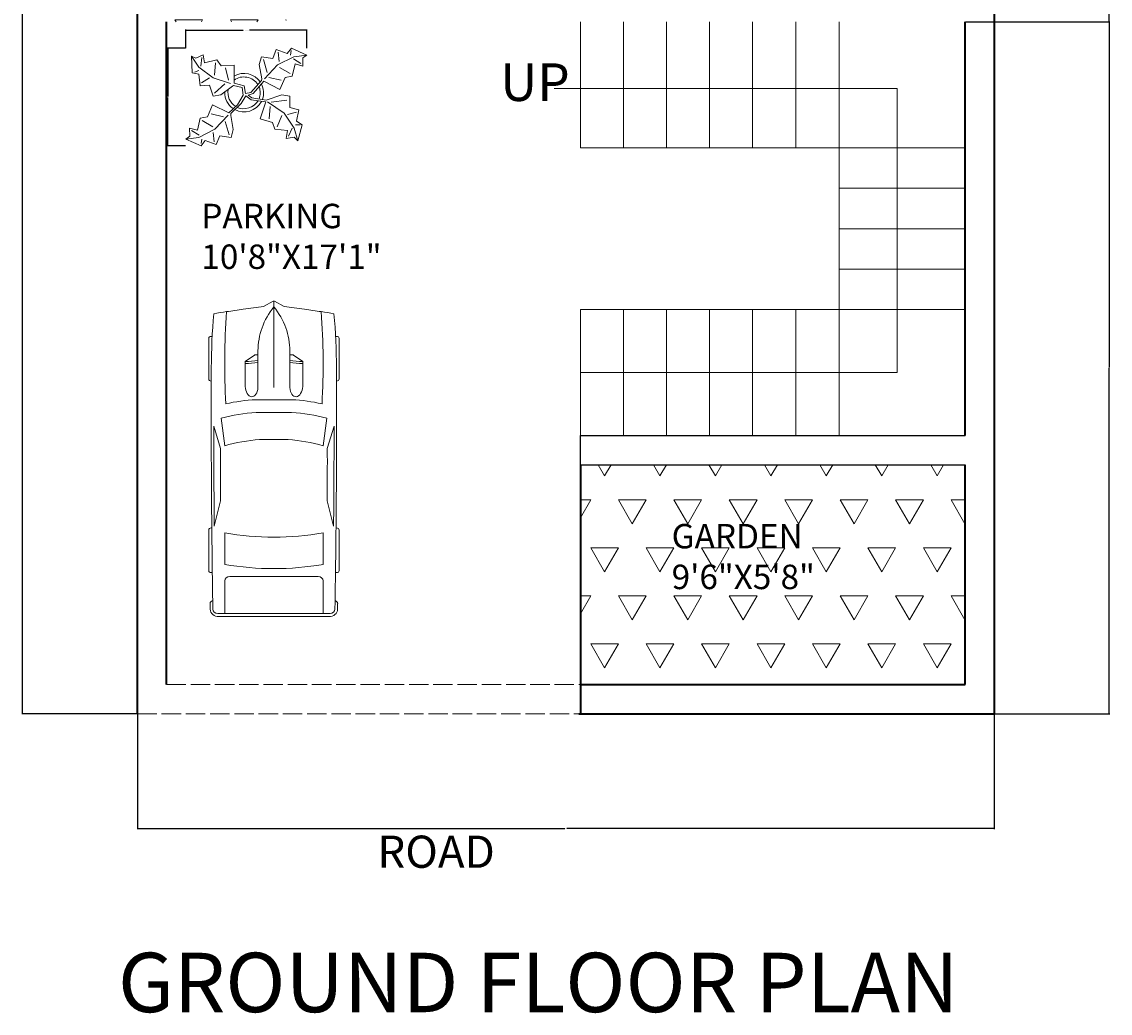
# Model space of a CAD drawing. Units: inches. Extents: x 7766 to 8631, y 9203 to 9940.
# Tile 1 of 6: x 7766 to 8103, y 9203 to 9510. Entities that reach past the tile are written whole.
import ezdxf

# ---------------------------------------------------------------- set-up
doc = ezdxf.new("R2010")
doc.units = ezdxf.units.IN
doc.linetypes.add('ACAD_ISO02W100', pattern=[15, 12, -3])
for name, color, linetype, lineweight in [('A-ANNO-DIMS', 2, 'Continuous', 18), ('A-ANNO-TEXT', 7, 'Continuous', 18), ('A-AREA-IDEN', 11, 'Continuous', 18), ('A-WALL', 7, 'Continuous', 35), ('C-SITE-ENTR', 7, 'ACAD_ISO02W100', 18), ('car', 20, 'Continuous', 13), ('floor', 7, 'Continuous', 25), ('flower', 70, 'Continuous', 18), ('L-PLNT-PATT', 60, 'Continuous', 13), ('stair', 2, 'Continuous', 18), ('TITLE', 4, 'Continuous', 35)]:
    doc.layers.add(name, color=color, linetype=linetype, lineweight=lineweight)
doc.styles.get("Standard").update_dxf_attribs({"font": 'arial.ttf'})
doc.dimstyles.get("Standard").update_dxf_attribs({"dimtxt": 0.18, "dimasz": 0.18, "dimexe": 0.18, "dimexo": 0.0625, "dimgap": 0.09, "dimtad": 0, "dimtih": 1, "dimtoh": 1, "dimdec": 4, "dimzin": 0, "dimdsep": 46, "dimtxsty": 'Standard', "dimcen": 0.09, "dimadec": 0, "dimazin": 0, "dimtfac": 1, "dimtdec": 4, "dimtofl": 0, "dimtmove": 0, "dimatfit": 3, "dimfxl": 1, "dimtolj": 1, "dimtzin": 0, "dimarcsym": 0})

# ---------------------------------------------------------------- blocks, each defined once
blk = doc.blocks.new('Plant - Rubber or Philodendron')
for p, q in [((8.8871, 10.7908), (9.9809, 13.4933)), ((9.9809, 13.4933), (13.3837, 12.301)), ((13.3837, 12.301), (14.68, 13.9039)), ((14.68, 13.9039), (19.3848, 11.8146)), ((-16.2005, 11.4774), (-13.9899, 8.1064)), ((-16.2005, 11.4774), (-14.8639, 10.7964)), ((-16.0159, 6.3329), (-16.2005, 11.4774)), ((-14.8639, 10.7964), (-12.6195, 11.8975)), ((-13.3174, 8.325), (-13.0735, 11.0065)), ((-12.6195, 11.8975), (-12.1909, 9.4345)), ((-12.1909, 9.4345), (-8.3829, 10.3)), ((-8.3829, 10.3), (-7.0549, 8.501)), ((4.6914, 8.8812), (5.3859, 11.2828)), ((5.3859, 11.2828), (8.8871, 10.7908)), ((5.9878, 10.4842), (7.1971, 6.3869)), ((15.3859, 11.3055), (10.3916, 8.7942)), ((10.5828, 12.6946), (10.8893, 9.7953)), ((14.5816, 13.2037), (14.3848, 11.8033)), ((15.2875, 10.6053), (17.5907, 9.2105)), ((19.3848, 11.8146), (15.3859, 11.3055)), ((19.3848, 11.8146), (18.1868, 10.9119)), ((18.1868, 10.9119), (18.1925, 8.4119)), ((-15.3434, 6.5514), (-13.9984, 6.9884)), ((-13.9899, 8.1064), (-9.5434, 4.7185)), ((-8.8369, 9.409), (-9.0894, 5.6095)), ((-7.0549, 8.501), (-3.0284, 8.6941)), ((-4.8529, 4.012), (-5.7184, 7.82)), ((-3.0284, 8.6941), (-3.0709, 3.1041)), ((4.6914, 8.8812), (5.5014, 4.4831)), ((10.3916, 8.7942), (6.2847, 4.4028)), ((14.2977, 6.1031), (10.9934, 7.9956)), ((15.7909, 9.1065), (14.8995, 5.3044)), ((18.1925, 8.4119), (15.7909, 9.1065)), ((-14.0069, 5.8704), (-16.0159, 6.3329)), ((-13.5868, 2.2894), (-14.0069, 5.8704)), ((-13.1329, 3.1804), (-10.6614, 4.727)), ((-9.5434, 4.7185), (-4.1917, 2.9888)), ((2.1141, 0.2298), (5.4346, 3.9146)), ((6.1032, 3.6844), (2.8262, -0.031)), ((5.4346, 3.9146), (5.5014, 4.4831)), ((11.1089, 1.1958), (6.1032, 3.6844)), ((7.7005, 4.8881), (11.5025, 3.9967)), ((12.7005, 4.8994), (11.1089, 1.1958)), ((14.8995, 5.3044), (12.7005, 4.8994)), ((-10.6784, 2.491), (-13.5868, 2.2894)), ((-9.5858, -0.8715), (-10.6784, 2.491)), ((-9.1318, 0.0195), (-5.9793, 2.9025)), ((-7.1228, -0.443), (-3.5248, 2.2131)), ((-3.5248, 2.2131), (-3.3011, 2.4355)), ((-3.3011, 2.4355), (-0.5306, 1.7947)), ((-3.0709, 3.1041), (0.0797, 2.3163)), ((-0.5306, 1.7947), (-0.2255, -0.5527)), ((-0.5306, 1.7947), (-0.5306, 1.7947)), ((0.0797, 2.3163), (0.4866, -0.031)), ((0.4866, -0.031), (2.1141, 0.2298)), ((-7.1228, -0.443), (-9.5858, -0.8715)), ((-4.0579, -6.2781), (-0.9375, -3.1608)), ((-2.019, -3.6148), (-0.2255, -0.5527)), ((-0.9375, -3.1608), (0.5883, -0.8135)), ((0.5883, -0.8135), (2.2447, -2.0916)), ((2.8262, -0.031), (1.3003, -0.5527)), ((1.3003, -0.5527), (2.4193, -1.4655)), ((2.2447, -2.0916), (6.7108, -2.6626)), ((2.4193, -1.4655), (6.895, -2.1175)), ((4.943, -7.9659), (6.7108, -2.6626)), ((11.6605, -0.5413), (6.895, -2.1175)), ((12.3677, -6.1981), (7.219, -2.6772)), ((8.3544, -2.7453), (13.1973, -2.1704)), ((11.6605, -0.5413), (14.1354, -0.8948)), ((14.1354, -0.8948), (14.1354, -4.4304)), ((-11.3237, -7.2629), (-9.7321, -3.5593)), ((-6.3237, -7.2516), (-10.1257, -6.3602)), ((-9.7321, -3.5593), (-4.7264, -6.0479)), ((-2.019, -3.6148), (-4.7264, -6.0479)), ((-4.1246, -6.8466), (-4.0579, -6.2781)), ((8.125, -4.0768), (7.7715, -7.9659)), ((15.5496, -10.7943), (12.3677, -6.1981)), ((16.2567, -5.8446), (13.4283, -6.5517)), ((14.1354, -4.4304), (16.9638, -5.1375)), ((16.9638, -5.1375), (16.2567, -8.673)), ((-14.4141, -11.4699), (-13.5228, -7.6679)), ((-13.5228, -7.6679), (-11.3237, -7.2629)), ((-12.921, -8.4665), (-9.6166, -10.359)), ((-9.0148, -11.1577), (-4.9047, -6.8122)), ((-4.611, -12.8477), (-5.8203, -8.7504)), ((-3.3146, -11.2447), (-4.1246, -6.8466)), ((8.8321, -9.0266), (4.943, -7.9659)), ((9.5392, -11.1479), (8.8321, -9.0266)), ((10.2463, -10.4408), (11.6605, -6.9053)), ((17.3174, -9.7337), (15.9032, -9.7337)), ((16.2567, -8.673), (18.0245, -9.7337)), ((18.0245, -9.7337), (16.6103, -14.6834)), ((-18.008, -14.1781), (-16.8101, -13.2754)), ((-16.8157, -10.7754), (-14.4141, -11.4699)), ((-16.8101, -13.2754), (-16.8157, -10.7754)), ((-13.9107, -12.9688), (-16.2139, -11.574)), ((-14.0091, -13.669), (-9.0148, -11.1577)), ((-9.206, -15.0581), (-9.5126, -12.1588)), ((-7.5103, -13.1543), (-8.6042, -15.8568)), ((-4.0092, -13.6463), (-7.5103, -13.1543)), ((-3.3146, -11.2447), (-4.0092, -13.6463)), ((13.4283, -11.5015), (9.5392, -11.1479)), ((13.0748, -13.9763), (13.4283, -11.5015)), ((14.8425, -10.7943), (13.7819, -13.2692)), ((16.6103, -14.6834), (15.5496, -10.7943)), ((-18.008, -14.1781), (-14.0091, -13.669)), ((-13.3032, -16.2674), (-18.008, -14.1781)), ((-12.0069, -14.6645), (-13.3032, -16.2674)), ((-13.2048, -15.5672), (-13.008, -14.1668)), ((-8.6042, -15.8568), (-12.0069, -14.6645)), ((15.5496, -13.6228), (13.0748, -13.9763)), ((16.6103, -14.6834), (15.5496, -13.6228))]:
    blk.add_line(p, q)
for centre, radius, start, end in [((0, 0), 6.1275, 34.37569, 120.1028), ((-0.0601, -0.2075), 5.2461, 33.82192, 124.9414), ((0.0308, 0.1664), 6, 178.6147, 235.1169), ((0.0308, 0.1664), 5, 168.1647, 238.6725), ((-0.2664, 0.1682), 5.2775, 338.4094, 20.03007), ((-0.098, 0.1364), 6.1288, 341.2017, 26.09184), ((-0.0234, 0.3825), 6.1492, 242.5812, 331.2714), ((-0.1102, 0.4886), 5.2883, 247.3711, 327.472)]:
    blk.add_arc(centre, radius, start, end)
blk = doc.blocks.new('*U22')
for p, q in [((21.1, 37.41), (21.1, 36.83)), ((46.55, 38.89), (22.35, 38.89)), ((47.8, 37.39), (47.8, 37.41)), ((87.99, 31.87), (74.76, 35.92)), ((134.31, 35.6), (119.29, 31.78)), ((135.45, 37.07), (135.45, 37.41)), ((136.7, 38.89), (160.9, 38.89)), ((162.15, 37.41), (162.15, 36.77)), ((186.47, -33.5), (186.47, 33.5)), ((188.4, -32.76), (188.4, 32.76)), ((70.03, 31.54), (86.41, 29.35)), ((138.42, 29.35), (157.25, 29.35)), ((164.52, 26.39), (164.52, -26.39)), ((186.47, 29.35), (167.01, 29.35)), ((32.27, 11.63), (36.13, 17.17)), ((36.13, 17.17), (50.94, 17.17)), ((29.77, 9.51), (51.68, 9.51)), ((32.12, 9.51), (32.12, 11.15)), ((58.92, -10.77), (58.92, 10.77)), ((66.55, -10.53), (66.55, 10.53)), ((82.74, 8.5), (82.74, -8.5)), ((186.47, -10.53), (186.47, 10.53)), ((3.27, 6.13), (0.1, 0.41)), ((0, 0), (51.68, 0)), ((0.1, -0.41), (3.27, -6.13)), ((29.77, -9.51), (51.68, -9.51)), ((32.12, -9.51), (32.12, -11.15)), ((32.27, -11.63), (36.13, -17.17)), ((36.13, -17.17), (50.94, -17.17)), ((86.41, -29.35), (70.03, -31.54)), ((87.99, -31.87), (74.76, -35.92)), ((134.31, -35.6), (119.29, -31.78)), ((157.25, -29.35), (138.42, -29.35)), ((167.01, -29.35), (186.47, -29.35)), ((21.1, -37.41), (21.1, -36.83)), ((46.55, -38.89), (22.35, -38.89)), ((47.8, -37.39), (47.8, -37.41)), ((135.45, -37.07), (135.45, -37.41)), ((136.7, -38.89), (160.9, -38.89)), ((162.15, -37.41), (162.15, -36.77))]:
    blk.add_line(p, q)
for centre, major_axis, ratio, start_param, end_param in [((266.03, -27.52), (0, 313.31), 0.842304, 1.367076, 1.39176), ((41.19, -490.86), (0, 528.23), 0.842304, 0.00281, 0.075598), ((22.35, 37.41), (0, -1.48), 0.842304, 3.141593, 4.712389), ((64.48, -10555.62), (0, 10593.03), 0.842304, -0.013397, 0.002797), ((46.55, 37.41), (0, 1.48), 0.842304, -1.570796, 0), ((64.48, -10555.62), (0, -10591.55), 0.842304, 3.133765, 3.140441), ((136.7, 37.41), (0, -1.48), 0.842304, 3.141593, 4.712389), ((160.9, 37.41), (0, 1.48), 0.842304, -1.570796, 0), ((180.63, 35.84), (0, 2.22), 0.842304, -0.013017, 1.249894), ((64.48, -10556.36), (0, 10595.31), 0.842304, -0.013397, -0.013017), ((183.98, 33.5), (0, -2.96), 0.842304, 1.570796, 3.128196), ((183.98, 32.76), (0, -5.25), 0.842304, 1.570796, 3.128196), ((259.18, -27.52), (0, -305.3), 0.842304, 4.528606, 4.561838), ((37.47, -593.96), (0, -623.33), 0.842304, 3.096046, 3.200911), ((134.4, 5.39), (0, -89.78), 0.842304, 4.449482, 4.652344), ((135.29, 5.39), (0, 81.77), 0.842304, 1.245306, 1.50788), ((149.6, 2.8), (0, -79.58), 0.842304, 4.372215, 4.640744), ((95.79, -3666.35), (0, -3698.24), 0.842304, 3.134049, 3.144098), ((17.08, 0), (0, 147.02), 0.842304, 4.511394, 4.913384), ((35.91, 0), (0, 147.02), 0.842304, 4.511394, 4.913384), ((167.01, 26.39), (0, 2.96), 0.842304, 0, 1.570796), ((-204.49, 52.4), (0, -250.96), 0.842304, 1.385369, 1.434372), ((13.04, 17.01), (0, 27.42), 0.842304, 4.435146, 4.718221), ((14.2, 17.01), (0, 27.42), 0.842304, 4.435146, 4.718221), ((50.79, 13.34), (6.34, -0.36), 0.603834, -1.395552, 1.581315), ((29.77, -46.66), (0, 56.17), 0.842304, 0, 0.590319), ((32.75, 11.15), (0, 0.74), 0.842304, 0.879714, 1.570796), ((0.62, 0), (0, -0.74), 0.842304, 4.131459, 5.293319), ((-204.49, -52.4), (0, 250.96), 0.842304, -1.434372, -1.385369), ((29.77, 46.66), (0, 56.17), 0.842304, 2.551274, 3.141593), ((32.75, -11.15), (0, -0.74), 0.842304, 4.712389, 5.403472), ((13.04, -17.01), (0, -27.42), 0.842304, 1.564964, 1.848039), ((14.2, -17.01), (0, -27.42), 0.842304, 1.564964, 1.848039), ((134.4, -5.39), (0, -89.78), 0.842304, -1.510751, -1.307889), ((135.29, -5.39), (0, -81.77), 0.842304, -1.50788, -1.245306), ((149.6, -2.8), (0, -79.58), 0.842304, -1.499151, -1.230623), ((259.18, 27.52), (0, 305.3), 0.842304, 1.721348, 1.754579), ((266.03, 27.52), (0, 313.31), 0.842304, 1.749832, 1.774517), ((37.47, 593.96), (0, -623.33), 0.842304, -0.059319, 0.045547), ((95.79, 3666.35), (0, -3698.24), 0.842304, -0.002505, 0.007544), ((167.01, -26.39), (0, -2.96), 0.842304, 4.712389, 6.283185), ((41.19, 490.86), (0, -528.23), 0.842304, -0.075598, -0.00281), ((22.35, -37.41), (0, 1.48), 0.842304, 1.570796, 3.141593), ((64.48, 10555.62), (0, 10593.03), 0.842304, 3.138796, 3.15499), ((46.55, -37.41), (0, -1.48), 0.842304, 0, 1.570796), ((64.48, 10555.62), (0, -10591.55), 0.842304, 0.001152, 0.007828), ((136.7, -37.41), (0, -1.48), 0.842304, -1.570796, 0), ((160.9, -37.41), (0, 1.48), 0.842304, 3.141593, 4.712389), ((180.63, -35.84), (0, -2.22), 0.842304, -1.249894, 0.013017), ((64.48, 10556.36), (0, 10595.31), 0.842304, 3.15461, 3.15499), ((183.98, -33.5), (0, 2.96), 0.842304, 3.15499, 4.712389), ((183.98, -32.76), (0, -5.25), 0.842304, 0.013397, 1.570796)]:
    blk.add_ellipse(centre, major_axis=major_axis, ratio=ratio, start_param=start_param, end_param=end_param)
at = {"extrusion": (0, 0, -1)}
blk.add_ellipse((50.79, -13.34), major_axis=(6.34, 0.36), ratio=0.603834, start_param=-1.395552, end_param=1.581315, dxfattribs=at)
blk = doc.blocks.new('STAIR-U-RETURN')
for p, q in [((8.13, 89), (8.13, 128)), ((21.45, 89), (21.45, 128)), ((34.76, 89), (34.76, 128)), ((48.08, 89), (48.08, 128)), ((61.39, 89), (61.39, 128)), ((74.71, 89), (74.71, 128)), ((88.13, 0), (88.13, 128)), ((0, 107.36), (106.07, 107.36)), ((106.07, 107.36), (106.07, 19.51)), ((13.13, 89), (8.13, 89)), ((13.13, 89), (88.13, 89)), ((88.13, 89), (127.13, 89)), ((88.13, 76.5), (127.13, 76.5)), ((88.13, 64), (127.13, 64)), ((88.13, 51.5), (127.13, 51.5)), ((8.13, 39), (88.13, 39)), ((8.13, 39), (8.13, 0)), ((21.45, 39), (21.45, 0)), ((34.76, 39), (34.76, 0)), ((48.08, 39), (48.08, 0)), ((61.39, 39), (61.39, 0)), ((74.71, 39), (74.71, 0)), ((88.13, 39), (127.13, 39)), ((106.07, 19.51), (8.13, 19.5))]:
    blk.add_line(p, q)
blk = doc.blocks.new('*D58')
at = {"layer": 'A-ANNO-DIMS', "color": 0, "lineweight": -2, "transparency": 16777216}
for p, q in [((7817.22, 9501.43), (7817.22, 9507.15)), ((7817.4, 9506.97), (7834.95, 9506.97)), ((7854.43, 9506.97), (7836.88, 9506.97)), ((7854.61, 9501.43), (7854.61, 9507.15))]:
    blk.add_line(p, q, dxfattribs=at)
at = {"layer": 'A-ANNO-DIMS', "color": 0, "transparency": 16777216}
for points in [[(7817.4, 9507), (7817.4, 9506.94), (7817.22, 9506.97)], [(7854.43, 9507), (7854.43, 9506.94), (7854.61, 9506.97)]]:
    blk.add_solid(points, dxfattribs=at)
at = {"layer": 'Defpoints', "color": 0, "transparency": 16777216}
for p in [(7854.61, 9506.97), (7817.22, 9501.36), (7854.61, 9501.36)]:
    blk.add_point(p, dxfattribs=at)
at = {"layer": 'A-ANNO-DIMS', "color": 0, "transparency": 16777216, "insert": (7835.91, 9506.97), "char_height": 0.18, "attachment_point": 5}
blk.add_mtext('\\A1;PLANT 37 TYP.', dxfattribs=at)
blk = doc.blocks.new('*D59')
at = {"layer": 'A-ANNO-DIMS', "color": 0, "lineweight": -2, "transparency": 16777216}
for p, q in [((7817.15, 9501.36), (7811.43, 9501.36)), ((7811.61, 9501.18), (7811.61, 9486.46)), ((7811.61, 9471.37), (7811.61, 9486.1)), ((7817.15, 9471.19), (7811.43, 9471.19))]:
    blk.add_line(p, q, dxfattribs=at)
at = {"layer": 'A-ANNO-DIMS', "color": 0, "transparency": 16777216}
for points in [[(7811.58, 9501.18), (7811.64, 9501.18), (7811.61, 9501.36)], [(7811.58, 9471.37), (7811.64, 9471.37), (7811.61, 9471.19)]]:
    blk.add_solid(points, dxfattribs=at)
at = {"layer": 'Defpoints', "color": 0, "transparency": 16777216}
for p in [(7811.61, 9501.36), (7817.22, 9501.36), (7817.22, 9471.19)]:
    blk.add_point(p, dxfattribs=at)
at = {"layer": 'A-ANNO-DIMS', "color": 0, "transparency": 16777216, "insert": (7811.61, 9486.28), "char_height": 0.18, "attachment_point": 5}
blk.add_mtext('\\A1;30 TYP.', dxfattribs=at)
blk = doc.blocks.new('*D68')
at = {"layer": 'A-ANNO-DIMS', "color": 0, "lineweight": -2, "transparency": 16777216}
for p, q in [((7802.24, 9295.5), (7802.24, 9259.83)), ((8067.24, 9295.5), (8067.24, 9259.83)), ((7802.42, 9260.01), (7934.45, 9260.01)), ((8067.06, 9260.01), (7935.03, 9260.01))]:
    blk.add_line(p, q, dxfattribs=at)
at = {"layer": 'A-ANNO-DIMS', "color": 0, "transparency": 16777216}
for points in [[(7802.42, 9260.04), (7802.42, 9259.98), (7802.24, 9260.01)], [(8067.06, 9260.04), (8067.06, 9259.98), (8067.24, 9260.01)]]:
    blk.add_solid(points, dxfattribs=at)
at = {"layer": 'Defpoints', "color": 0, "transparency": 16777216}
for p in [(7802.24, 9295.56), (8067.24, 9295.56), (8067.24, 9260.01)]:
    blk.add_point(p, dxfattribs=at)
at = {"layer": 'A-ANNO-DIMS', "color": 0, "transparency": 16777216, "insert": (7934.74, 9260.01), "char_height": 0.18, "attachment_point": 5}
blk.add_mtext('\\A1;265', dxfattribs=at)
blk = doc.blocks.new('*D69')
at = {"layer": 'A-ANNO-DIMS', "color": 0, "lineweight": -2, "transparency": 16777216}
for p, q in [((7802.18, 9904.56), (7766.51, 9904.56)), ((7766.69, 9904.38), (7766.69, 9600.25)), ((7766.69, 9295.74), (7766.69, 9599.88)), ((7802.18, 9295.56), (7766.51, 9295.56))]:
    blk.add_line(p, q, dxfattribs=at)
at = {"layer": 'A-ANNO-DIMS', "color": 0, "transparency": 16777216}
for points in [[(7766.66, 9904.38), (7766.72, 9904.38), (7766.69, 9904.56)], [(7766.66, 9295.74), (7766.72, 9295.74), (7766.69, 9295.56)]]:
    blk.add_solid(points, dxfattribs=at)
at = {"layer": 'Defpoints', "color": 0, "transparency": 16777216}
for p in [(7766.69, 9904.56), (7802.24, 9904.56), (7802.24, 9295.56)]:
    blk.add_point(p, dxfattribs=at)
at = {"layer": 'A-ANNO-DIMS', "color": 0, "transparency": 16777216, "insert": (7766.69, 9600.06), "char_height": 0.18, "attachment_point": 5}
blk.add_mtext('\\A1;609', dxfattribs=at)
blk = doc.blocks.new('*D72')
at = {"layer": 'A-ANNO-DIMS', "color": 0, "lineweight": -2, "transparency": 16777216}
for p, q in [((8058.31, 9509.56), (8102.97, 9509.56)), ((8102.79, 9509.38), (8102.79, 9402.74)), ((8102.79, 9295.74), (8102.79, 9402.38)), ((8067.31, 9295.56), (8102.97, 9295.56))]:
    blk.add_line(p, q, dxfattribs=at)
at = {"layer": 'A-ANNO-DIMS', "color": 0, "transparency": 16777216}
for points in [[(8102.76, 9509.38), (8102.82, 9509.38), (8102.79, 9509.56)], [(8102.76, 9295.74), (8102.82, 9295.74), (8102.79, 9295.56)]]:
    blk.add_solid(points, dxfattribs=at)
at = {"layer": 'Defpoints', "color": 0, "transparency": 16777216}
for p in [(8058.24, 9509.56), (8102.79, 9509.56), (8067.24, 9295.56)]:
    blk.add_point(p, dxfattribs=at)
at = {"layer": 'A-ANNO-DIMS', "color": 0, "transparency": 16777216, "insert": (8102.79, 9402.56), "char_height": 0.18, "attachment_point": 5}
blk.add_mtext('\\A1;214', dxfattribs=at)
blk = doc.blocks.new('*D81')
at = {"layer": 'A-ANNO-DIMS', "color": 0, "lineweight": -2, "transparency": 16777216}
for p, q in [((8067.31, 9551.3), (8102.97, 9551.3)), ((8102.79, 9551.12), (8102.79, 9530.61)), ((8102.79, 9509.74), (8102.79, 9530.25)), ((8058.31, 9509.56), (8102.97, 9509.56))]:
    blk.add_line(p, q, dxfattribs=at)
at = {"layer": 'A-ANNO-DIMS', "color": 0, "transparency": 16777216}
for points in [[(8102.76, 9551.12), (8102.82, 9551.12), (8102.79, 9551.3)], [(8102.76, 9509.74), (8102.82, 9509.74), (8102.79, 9509.56)]]:
    blk.add_solid(points, dxfattribs=at)
at = {"layer": 'Defpoints', "color": 0, "transparency": 16777216}
for p in [(8067.24, 9551.3), (8102.79, 9551.3), (8058.24, 9509.56)]:
    blk.add_point(p, dxfattribs=at)
at = {"layer": 'A-ANNO-DIMS', "color": 0, "transparency": 16777216, "insert": (8102.79, 9530.43), "char_height": 0.18, "attachment_point": 5}
blk.add_mtext('\\A1;41.73', dxfattribs=at)

msp = doc.modelspace()

# ---------------------------------------------------------------- hatches: boundary and pattern name
at = {"layer": 'L-PLNT-PATT'}
h = msp.add_hatch(dxfattribs=at)
h.set_pattern_fill('TRIANG', color=256, scale=1.8)
h.paths.add_polyline_path([(7848.243, 9895.5631), (7811.243, 9895.5631), (7811.243, 9784.5631), (7848.243, 9784.5631)])
h.paths.add_polyline_path([(7848.243, 9655.5631), (7811.243, 9655.5631), (7811.243, 9509.5631), (7848.243, 9509.5631)])
h.paths.add_polyline_path([(8058.243, 9372.5631), (7939.243, 9372.5631), (7939.243, 9304.5631), (8058.243, 9304.5631)])
h.paths.add_polyline_path([(7817.6934, 9855.8718), (7817.6934, 9803.4053), (7845.8896, 9803.4053), (7845.8896, 9855.8718)], flags=24)
h.paths.add_polyline_path([(7814.5059, 9594.625), (7814.5059, 9542.1584), (7842.7021, 9542.1584), (7842.7021, 9594.625)], flags=24)
h.paths.add_polyline_path([(7965.0141, 9329.808), (8013.9551, 9329.808), (8013.9551, 9358.0042), (7965.0141, 9358.0042)], flags=24)

# ---------------------------------------------------------------- linework, layer by layer
at = {"layer": 'A-WALL'}
for p, q in [((7802.243, 9295.5631), (7802.243, 9904.5631)), ((8067.243, 9895.5631), (8067.243, 9295.5631)), ((7811.243, 9304.5631), (7811.243, 9509.5631)), ((8058.243, 9381.5631), (8058.243, 9509.5631)), ((7939.243, 9372.5631), (7939.243, 9295.5631)), ((8058.243, 9304.5631), (8058.243, 9372.5631)), ((7939.243, 9304.5631), (8058.243, 9304.5631)), ((7944.243, 9304.5631), (8000.243, 9304.5631)), ((7938.7785, 9295.5631), (8067.243, 9295.5631))]:
    msp.add_line(p, q, dxfattribs=at)
at = {"layer": 'C-SITE-ENTR', "ltscale": 0.5}
for p, q in [((7811.243, 9304.5631), (7939.243, 9304.5631)), ((7802.243, 9295.5631), (7938.7785, 9295.5631))]:
    msp.add_line(p, q, dxfattribs=at)
at = {"layer": 'floor'}
for p, q in [((7939.243, 9381.5631), (8058.243, 9381.5631)), ((7939.243, 9372.5631), (7939.243, 9381.5631)), ((7939.243, 9372.5631), (8058.243, 9372.5631))]:
    msp.add_line(p, q, dxfattribs=at)
at = {"layer": 'flower'}
msp.add_lwpolyline([(7939.243, 9372.5631), (8058.243, 9372.5631), (8058.243, 9304.5631), (7939.243, 9304.5631)], close=True, dxfattribs=at)

# ---------------------------------------------------------------- block references
at = {"layer": 'car', "xscale": 0.5181177062043194, "yscale": 0.5181177062043194, "zscale": 0.5181177062043194, "rotation": 270}
msp.add_blockref('*U22', (7844.4631, 9423.1958), dxfattribs=at)
at = {"layer": 'flower'}
msp.add_blockref('Plant - Rubber or Philodendron', (7835.2242, 9487.4593), dxfattribs=at)
at = {"layer": 'stair'}
msp.add_blockref('STAIR-U-RETURN', (7931.11, 9381.563), dxfattribs=at)

# ---------------------------------------------------------------- texts
at = {"layer": 'A-ANNO-TEXT'}
for s, height, p in [('UP', 11.64486, (7914.4511, 9485.0619)), ('ROAD', 9.95997, (7876.4633, 9247.8893))]:
    msp.add_text(s, height=height, dxfattribs=at).set_placement(p)
at = {"layer": 'A-AREA-IDEN', "attachment_point": 1}
for s, insert, char_height in [('PARKING \\P10\'8"X17\'1"', (7822.0222, 9453.2678), 7.556341), ('GARDEN\\P9\'6"X5\'8"', (7967.4651, 9354.2441), 7.55634)]:
    msp.add_mtext_dynamic_manual_height_columns(s, width=97.347002, gutter_width=18.8909, heights=[0], dxfattribs=dict(at, insert=insert, char_height=char_height))
at = {"layer": 'TITLE'}
msp.add_text('GROUND FLOOR PLAN', height=18.381464, dxfattribs=at).set_placement((7796.2413, 9203.2441))

# ---------------------------------------------------------------- dimensions: what is measured, and where the dimension line sits
at = {"layer": 'A-ANNO-DIMS'}
for base, p1, p2, override, picture, middle in [((7766.693, 9904.5631), (7802.243, 9295.5631), (7802.243, 9904.5631), {"dimdec": 0, "dimlfac": 1, "dimrnd": 0, "dimzin": 0, "dimdsep": 46, "dimlunit": 2}, '*D69', (7766.693, 9600.0631)), ((8102.793, 9551.2962), (8058.243, 9509.5631), (8067.243, 9551.2962), {"dimdec": 2, "dimlfac": 1, "dimrnd": 0, "dimzin": 0, "dimdsep": 46, "dimlunit": 2}, '*D81', (8102.793, 9530.4296)), ((8102.793, 9509.5631), (8067.243, 9295.5631), (8058.243, 9509.5631), {"dimdec": 0, "dimlfac": 1, "dimrnd": 0, "dimzin": 0, "dimdsep": 46, "dimlunit": 2}, '*D72', (8102.793, 9402.5631))]:
    dim = msp.add_linear_dim(base=base, p1=p1, p2=p2, angle=90, dimstyle='Standard', override=override, dxfattribs=at)
    dim.commit()
    dim.dimension.update_dxf_attribs({"geometry": picture, "text_midpoint": middle})
dim = msp.add_linear_dim(base=(7854.609, 9506.9721), p1=(7817.2162, 9501.3632), p2=(7854.609, 9501.3632), text='PLANT <> TYP.', dimstyle='Standard', override={"dimdec": 0, "dimlfac": 1, "dimrnd": 0, "dimzin": 0, "dimdsep": 46, "dimlunit": 2}, dxfattribs=at)
dim.commit()
dim.dimension.update_dxf_attribs({"geometry": '*D58', "text_midpoint": (7835.9126, 9506.9721)})
dim = msp.add_linear_dim(base=(7811.6073, 9501.3632), p1=(7817.2162, 9471.1919), p2=(7817.2162, 9501.3632), angle=90, text='<> TYP.', dimstyle='Standard', override={"dimdec": 0, "dimlfac": 1, "dimrnd": 0, "dimzin": 0, "dimdsep": 46, "dimlunit": 2}, dxfattribs=at)
dim.commit()
dim.dimension.update_dxf_attribs({"geometry": '*D59', "text_midpoint": (7811.6073, 9486.2776)})
dim = msp.add_linear_dim(base=(8067.243, 9260.0131), p1=(7802.243, 9295.5631), p2=(8067.243, 9295.5631), dimstyle='Standard', override={"dimdec": 0, "dimlfac": 1, "dimrnd": 0, "dimzin": 0, "dimdsep": 46, "dimlunit": 2}, dxfattribs=at)
dim.commit()
dim.dimension.update_dxf_attribs({"geometry": '*D68', "text_midpoint": (7934.743, 9260.0131)})

doc.saveas('drawing.dxf')
